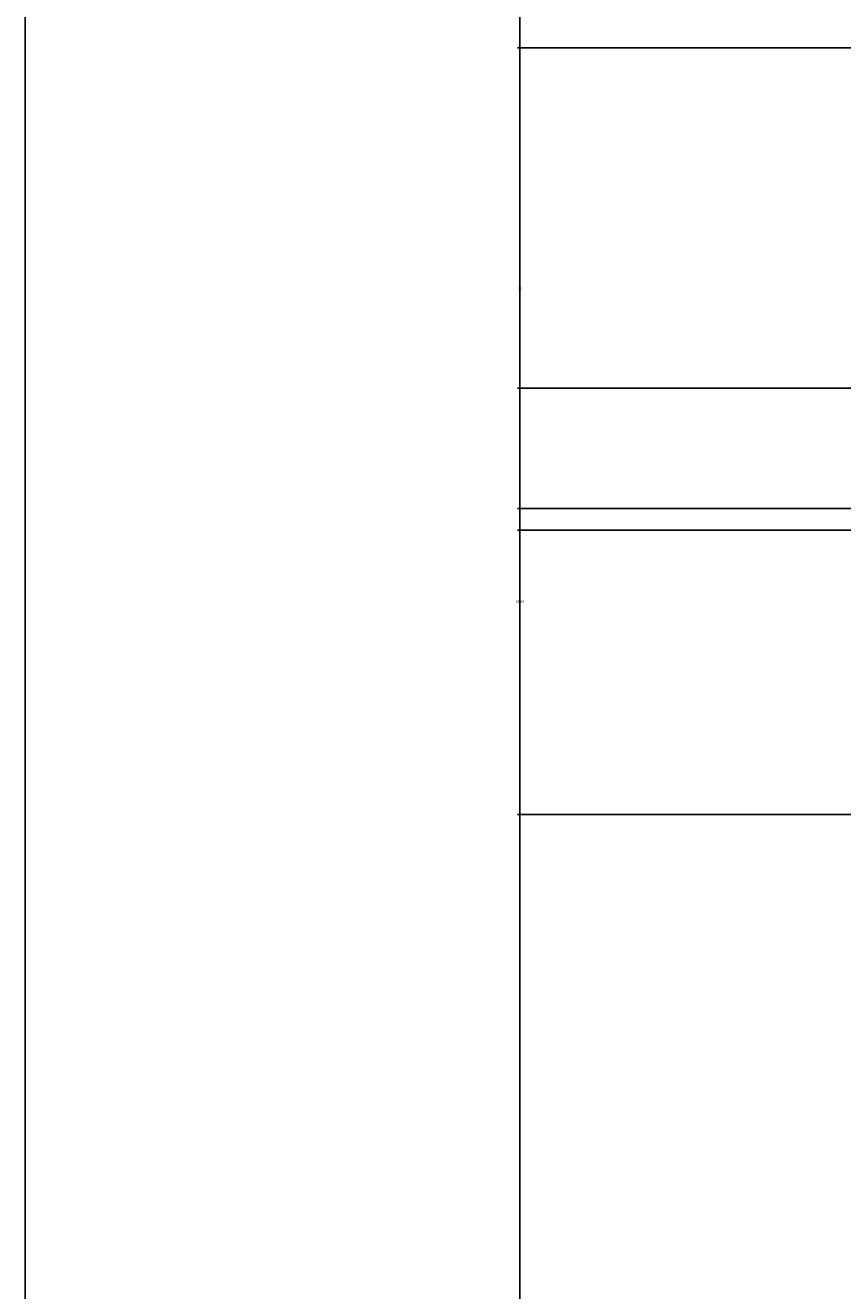
# Model space of a CAD drawing. Units: inches. Extents: x 1601 to 2297, y 1496 to 2631.
# Tile 9 of 57: x 1601 to 1662, y 1973 to 2067. Entities that reach past the tile are written whole.
import ezdxf

# ---------------------------------------------------------------- set-up
doc = ezdxf.new("R2010")
doc.units = ezdxf.units.IN
doc.layers.add('A-ANNO-DIMS', color=2, linetype='Continuous', lineweight=18)
doc.layers.add('A-ANNO-TTLB', color=7, linetype='Continuous', lineweight=25)
doc.styles.get("Standard").update_dxf_attribs({"font": 'arial.ttf'})
doc.dimstyles.get("Standard").update_dxf_attribs({"dimtxt": 0.18, "dimasz": 0.18, "dimexe": 0.18, "dimexo": 0.0625, "dimgap": 0.09, "dimtad": 0, "dimtih": 1, "dimtoh": 1, "dimdec": 4, "dimzin": 0, "dimdsep": 46, "dimtxsty": 'Standard', "dimcen": 0.09, "dimadec": 0, "dimazin": 0, "dimtfac": 1, "dimtdec": 4, "dimtofl": 0, "dimtmove": 0, "dimatfit": 3, "dimfxl": 1, "dimtolj": 1, "dimtzin": 0, "dimarcsym": 0})

# ---------------------------------------------------------------- blocks, each defined once
blk = doc.blocks.new('*D30')
at = {"layer": 'A-ANNO-DIMS', "color": 0, "lineweight": -2, "transparency": 16777216}
for p, q in [((1685.975, 2031.325), (1637.307, 2031.325)), ((1637.487, 2031.145), (1637.487, 1833.507)), ((1637.487, 1635.505), (1637.487, 1833.143)), ((1685.975, 1635.325), (1637.307, 1635.325))]:
    blk.add_line(p, q, dxfattribs=at)
at = {"layer": 'A-ANNO-DIMS', "color": 0, "transparency": 16777216}
for points in [[(1637.457, 2031.145), (1637.517, 2031.145), (1637.487, 2031.325)], [(1637.457, 1635.505), (1637.517, 1635.505), (1637.487, 1635.325)]]:
    blk.add_solid(points, dxfattribs=at)
at = {"layer": 'Defpoints', "color": 0, "transparency": 16777216}
for p in [(1637.487, 2031.325), (1686.037, 2031.325), (1686.037, 1635.325)]:
    blk.add_point(p, dxfattribs=at)
at = {"layer": 'A-ANNO-DIMS', "color": 0, "transparency": 16777216, "insert": (1637.487, 1833.325), "char_height": 0.18, "attachment_point": 5}
blk.add_mtext('\\A1;396', dxfattribs=at)
blk = doc.blocks.new('*D31')
at = {"layer": 'A-ANNO-DIMS', "color": 0, "lineweight": -2, "transparency": 16777216}
for p, q in [((1685.975, 2136.325), (1637.307, 2136.325)), ((1637.487, 2136.145), (1637.487, 2084.007)), ((1637.487, 2031.505), (1637.487, 2083.643)), ((1685.975, 2031.325), (1637.307, 2031.325))]:
    blk.add_line(p, q, dxfattribs=at)
at = {"layer": 'A-ANNO-DIMS', "color": 0, "transparency": 16777216}
for points in [[(1637.457, 2136.145), (1637.517, 2136.145), (1637.487, 2136.325)], [(1637.457, 2031.505), (1637.517, 2031.505), (1637.487, 2031.325)]]:
    blk.add_solid(points, dxfattribs=at)
at = {"layer": 'Defpoints', "color": 0, "transparency": 16777216}
for p in [(1637.487, 2136.325), (1686.037, 2136.325), (1686.037, 2031.325)]:
    blk.add_point(p, dxfattribs=at)
at = {"layer": 'A-ANNO-DIMS', "color": 0, "transparency": 16777216, "insert": (1637.487, 2083.825), "char_height": 0.18, "attachment_point": 5}
blk.add_mtext('\\A1;105', dxfattribs=at)
blk = doc.blocks.new('*D42')
at = {"layer": 'A-ANNO-DIMS', "color": 0, "lineweight": -2, "transparency": 16777216}
for p, q in [((2177.975, 2065.697), (1637.307, 2065.697)), ((1637.487, 2065.517), (1637.487, 2047.878)), ((1637.487, 2029.877), (1637.487, 2047.515)), ((2177.975, 2029.697), (1637.307, 2029.697))]:
    blk.add_line(p, q, dxfattribs=at)
at = {"layer": 'A-ANNO-DIMS', "color": 0, "transparency": 16777216}
for points in [[(1637.457, 2065.517), (1637.517, 2065.517), (1637.487, 2065.697)], [(1637.457, 2029.877), (1637.517, 2029.877), (1637.487, 2029.697)]]:
    blk.add_solid(points, dxfattribs=at)
at = {"layer": 'Defpoints', "color": 0, "transparency": 16777216}
for p in [(1637.487, 2065.697), (2178.037, 2065.697), (2178.037, 2029.697)]:
    blk.add_point(p, dxfattribs=at)
at = {"layer": 'A-ANNO-DIMS', "color": 0, "transparency": 16777216, "insert": (1637.487, 2047.697), "char_height": 0.18, "attachment_point": 5}
blk.add_mtext('\\A1;36', dxfattribs=at)
blk = doc.blocks.new('*D45')
at = {"layer": 'A-ANNO-DIMS', "color": 0, "lineweight": -2, "transparency": 16777216}
for p, q in [((1958.975, 2040.303), (1637.307, 2040.303)), ((1637.487, 2040.123), (1637.487, 2024.571)), ((1637.487, 2008.656), (1637.487, 2024.207)), ((1958.975, 2008.476), (1637.307, 2008.476))]:
    blk.add_line(p, q, dxfattribs=at)
at = {"layer": 'A-ANNO-DIMS', "color": 0, "transparency": 16777216}
for points in [[(1637.457, 2040.123), (1637.517, 2040.123), (1637.487, 2040.303)], [(1637.457, 2008.656), (1637.517, 2008.656), (1637.487, 2008.476)]]:
    blk.add_solid(points, dxfattribs=at)
at = {"layer": 'Defpoints', "color": 0, "transparency": 16777216}
for p in [(1637.487, 2040.303), (1959.037, 2040.303), (1959.037, 2008.476)]:
    blk.add_point(p, dxfattribs=at)
at = {"layer": 'A-ANNO-DIMS', "color": 0, "transparency": 16777216, "insert": (1637.487, 2024.389), "char_height": 0.18, "attachment_point": 5}
blk.add_mtext('\\A1;31.83', dxfattribs=at)

msp = doc.modelspace()

# ---------------------------------------------------------------- linework, layer by layer
at = {"layer": 'A-ANNO-TTLB'}
msp.add_lwpolyline([(1600.5933, 2631.1477), (2297.129, 2631.1477), (2297.129, 1496.1026), (1600.5933, 1496.1026)], close=True, dxfattribs=at)

# ---------------------------------------------------------------- dimensions: what is measured, and where the dimension line sits
at = {"layer": 'A-ANNO-DIMS'}
for base, p1, p2, override, picture, middle in [((1637.4873, 2136.3254), (1686.0373, 2031.3254), (1686.0373, 2136.3254), {"dimdec": 0, "dimlfac": 1, "dimrnd": 0, "dimzin": 0, "dimdsep": 46, "dimlunit": 2}, '*D31', (1637.4873, 2083.8254)), ((1637.4873, 2065.6965), (2178.0373, 2029.6965), (2178.0373, 2065.6965), {"dimdec": 0, "dimlfac": 1, "dimrnd": 0, "dimzin": 0, "dimdsep": 46, "dimlunit": 2}, '*D42', (1637.4873, 2047.6965)), ((1637.4873, 2040.3029), (1959.0373, 2008.4756), (1959.0373, 2040.3029), {"dimdec": 2, "dimlfac": 1, "dimrnd": 0, "dimzin": 0, "dimdsep": 46, "dimlunit": 2}, '*D45', (1637.4873, 2024.3893)), ((1637.4873, 2031.3254), (1686.0373, 1635.3254), (1686.0373, 2031.3254), {"dimdec": 0, "dimlfac": 1, "dimrnd": 0, "dimzin": 0, "dimdsep": 46, "dimlunit": 2}, '*D30', (1637.4873, 1833.3254))]:
    dim = msp.add_linear_dim(base=base, p1=p1, p2=p2, angle=90, dimstyle='Standard', override=override, dxfattribs=at)
    dim.commit()
    dim.dimension.update_dxf_attribs({"geometry": picture, "text_midpoint": middle})

doc.saveas('drawing.dxf')
